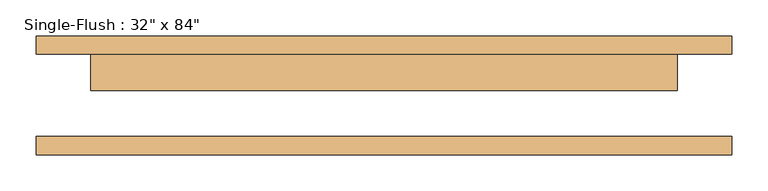
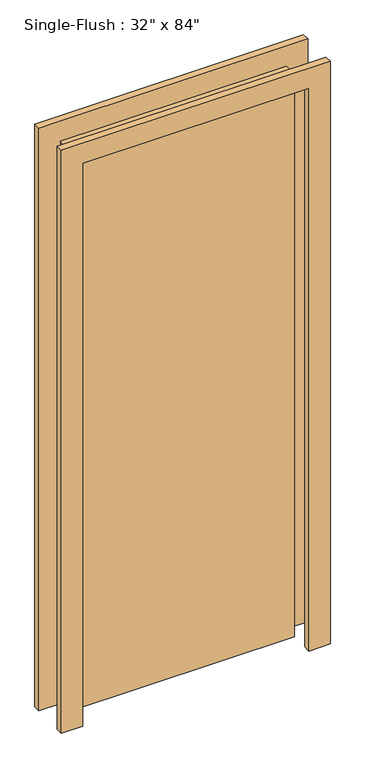
"""IFC4 building model written with IfcOpenShell, lengths in millimetres: door geometry."""

from ifc_helpers import new_model, si_unit, frame, origin, origin_with_axes, place, context, project, spatial, polyline, outline, extrude, source, transform, mapped, element, save


def door_d141acb4(model_context):
    return source(origin(), model_context, "Body", "SweptSolid", [
        extrude(outline(polyline([(2209.8, -482.6), (0.0, -482.6), (0.0, -406.4), (2133.6, -406.4), (2133.6, 406.4), (0.0, 406.4), (0.0, 482.6), (2209.8, 482.6), (2209.8, -482.6)])), frame((0.0, 57.15, 0.0), z_axis=(0.0, 1.0, 0.0), x_axis=(0.0, 0.0, 1.0)), (0.0, 0.0, 1.0), 25.4),
        extrude(outline(polyline([(2209.8, 482.6), (2209.8, -482.6), (0.0, -482.6), (0.0, -406.4), (2133.6, -406.4), (2133.6, 406.4), (0.0, 406.4), (0.0, 482.6), (2209.8, 482.6)])), frame((0.0, -82.55, 0.0), z_axis=(0.0, 1.0, 0.0), x_axis=(0.0, 0.0, 1.0)), (0.0, 0.0, 1.0), 25.4),
        extrude(outline(polyline([(406.4, 6.35), (-406.4, 6.35), (-406.4, 57.15), (406.4, 57.15), (406.4, 6.35)])), origin_with_axes(), (0.0, 0.0, 1.0), 2133.6),
    ])


if __name__ == "__main__":
    model = new_model("IFC4")
    model_context = context("Model", 3, world=origin())
    ifc_project = project(units=[si_unit("LENGTHUNIT", "METRE", prefix="MILLI")], contexts=[model_context])
    site = spatial("IfcSite", under=ifc_project)
    building = spatial("IfcBuilding", under=site)
    placement = place(None, origin())
    door_shape = door_d141acb4(model_context)
    element("IfcDoor", 1, ObjectType="Single-Flush : 32\" x 84\"", at=placement, inside=building, context=model_context, shape_type="MappedRepresentation", body=[
        mapped(door_shape, transform((0.0, 0.0, 0.0), x_axis=(1.0, 0.0, 0.0), y_axis=(0.0, 1.0, 0.0), z_axis=(0.0, 0.0, 1.0))),
    ])
    save(model, "model.ifc")

# Revit data of these elements
# Type "Single-Flush : 32\" x 84\""
#   Type Mark = "3"
#   Construction Type Id = "MDOOR"
#   Assembly Code = "C1020"
#   Analytic Construction = "Metal"
#   Thickness = 0' - 2"
#   Heat Transfer Coefficient (U) = 0.651978 BTU/(h·ft²·°F)
#   Height = 7' - 0"
#   Trim Projection Ext = 0' - 1"
#   Trim Projection Int = 0' - 1"
#   Trim Width = 0' - 3"
#   Width = 2' - 8"
#   Define Thermal Properties by = 1
#   Define Thermal Properties by = 1
#   Door Material = Door - Panel
#   Frame Material = Door - Frame
#   Visual Light Transmittance = 0
#   Solar Heat Gain Coefficient = 0
#   Function = (empty or 0)
#   Wall Closure = (empty or 0)
# Element 1 (IfcDoor, "Single-Flush : 32\" x 84\"")
#   Materials on its faces: "Door - Frame", "Door - Panel"
# Materials
#   "Door - Panel": class "Wood", colour RGB 210 159 95, transparency 0, Cost = 0
#   "Door - Frame": colour RGB 118 70 51, transparency 0, Cost = 0
